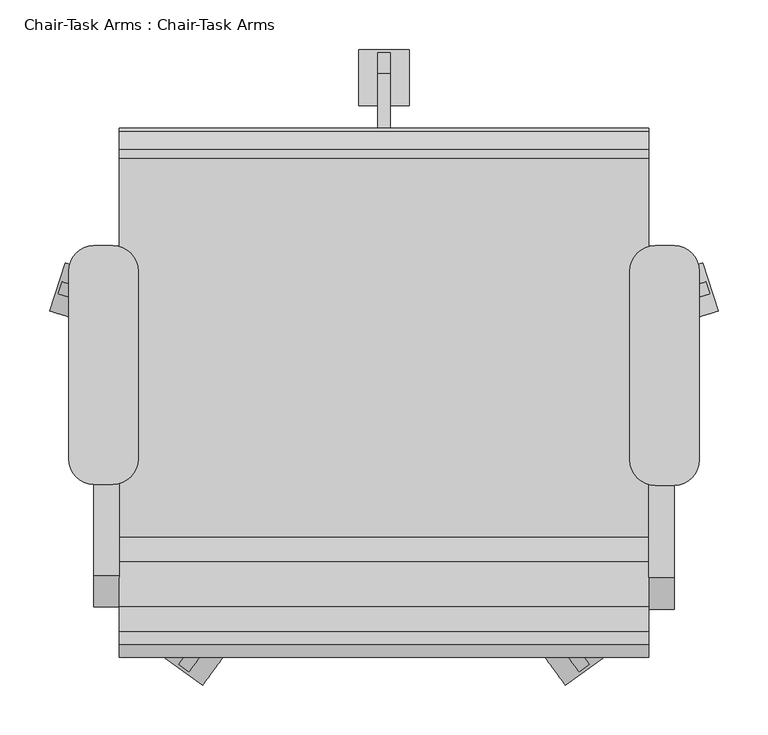
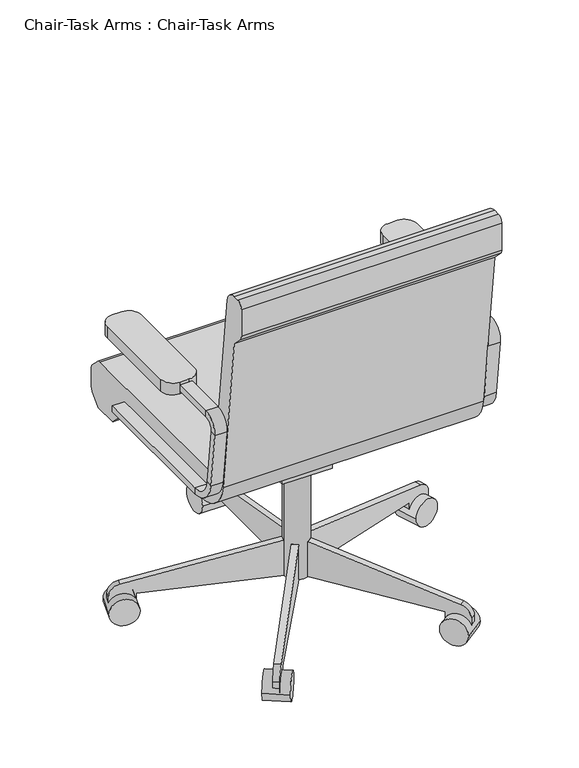
"""IFC4 building model written with IfcOpenShell, lengths in millimetres: furniture geometry, Chair-Task Arms : Chair-Task Arms."""

from ifc_helpers import new_model, si_unit, point, frame, frame_2d, origin, place, context, project, spatial, polyline, circle_curve, trimmed, segment, composite_curve, outline, extrude, source, transform, mapped, element, save
from ifc_brep_helpers import plane_surface, cylinder_surface, revolved_surface, advanced_brep


def chair_task_arms_chair_task_arms_bb362225(model_context):
    return source(origin(), model_context, "Body", "SolidModel", [
        extrude(outline(composite_curve([segment(polyline([(-126.2050455, 457.2), (255.0102301, 457.2)]), True, "CONTINUOUS"), segment(trimmed(circle_curve(frame_2d((255.0102301, 444.5)), 12.7), [point((255.0102301, 457.2))], [point((263.9604301, 453.510212))], False, "CARTESIAN"), True, "CONTINUOUS"), segment(polyline([(263.9604301, 453.510212), (281.8961016, 435.6939999)]), True, "CONTINUOUS"), segment(trimmed(circle_curve(frame_2d((272.9459016, 426.6837879)), 12.7), [point((281.8961016, 435.6939999))], [point((285.6459016, 426.6837879))], False, "CARTESIAN"), True, "CONTINUOUS"), segment(polyline([(285.6459016, 426.6837879), (285.6459016, 391.6405184)]), True, "CONTINUOUS"), segment(trimmed(circle_curve(frame_2d((260.2459016, 391.6405184)), 25.4), [point((285.6459016, 391.6405184))], [point((278.2663256, 373.7401184))], False, "CARTESIAN"), True, "CONTINUOUS"), segment(polyline([(278.2663256, 373.7401184), (260.2470284, 355.6), (209.4470284, 355.6), (181.0744602, 383.7835944), (-107.1089978, 383.7835944)]), True, "CONTINUOUS"), segment(trimmed(circle_curve(frame_2d((-107.1089978, 459.9835944)), 76.2), [point((-107.1089978, 383.7835944))], [point((-182.7870738, 451.0802913))], False, "CARTESIAN"), True, "CONTINUOUS"), segment(polyline([(-182.7870738, 451.0802913), (-222.3540984, 787.4), (-244.0343545, 809.0802561)]), True, "CONTINUOUS"), segment(trimmed(circle_curve(frame_2d((-235.0540984, 818.0605122)), 12.7), [point((-244.0343545, 809.0802561))], [point((-247.7540984, 818.0605122))], False, "CARTESIAN"), True, "CONTINUOUS"), segment(polyline([(-247.7540984, 818.0605122), (-247.7540984, 876.3)]), True, "CONTINUOUS"), segment(trimmed(circle_curve(frame_2d((-235.0540984, 876.3)), 12.7), [point((-247.7540984, 876.3))], [point((-235.0540984, 889.0))], False, "CARTESIAN"), True, "CONTINUOUS"), segment(polyline([(-235.0540984, 889.0), (-222.1789239, 889.0)]), True, "CONTINUOUS"), segment(trimmed(circle_curve(frame_2d((-222.1789239, 863.6)), 25.4), [point((-222.1789239, 889.0))], [point((-196.9528985, 866.5677677))], False, "CARTESIAN"), True, "CONTINUOUS"), segment(polyline([(-196.9528985, 866.5677677), (-151.4310708, 479.6322323)]), True, "CONTINUOUS"), segment(trimmed(circle_curve(frame_2d((-126.2050455, 482.6)), 25.4), [point((-151.4310708, 479.6322323))], [point((-126.2050455, 457.2))], True, "CARTESIAN"), True, "CONTINUOUS")], self_intersect=False)), frame((-125.7091803, 0.0, 0.0), z_axis=(1.0, 0.0, 0.0), x_axis=(0.0, 1.0, 0.0)), (0.0, 0.0, 1.0), 533.4),
        extrude(outline(polyline([(69.7459016, 383.7835944), (69.7459016, 371.0835944), (18.9459016, 283.0954134), (-19.1540984, 283.0954134), (-19.1540984, 383.7835944), (69.7459016, 383.7835944)])), frame((90.1908197, 0.0, 0.0), z_axis=(1.0, 0.0, 0.0), x_axis=(0.0, 1.0, 0.0)), (0.0, 0.0, 1.0), 101.6),
        extrude(outline(composite_curve([segment(polyline([(311.0459016, 53.5835944), (18.9459016, 53.5835944), (18.9459016, 129.7835944), (44.3459016, 129.7835944), (340.8565654, 77.5007643)]), True, "CONTINUOUS"), segment(trimmed(circle_curve(frame_2d((336.4459016, 52.4866474)), 25.4), [point((340.8565654, 77.5007643))], [point((361.8459016, 52.4866474))], False, "CARTESIAN"), True, "CONTINUOUS"), segment(polyline([(361.8459016, 52.4866474), (361.8459016, 28.1835944), (311.0459016, 28.1835944), (311.0459016, 53.5835944)]), True, "CONTINUOUS")], self_intersect=False)), frame((134.6408197, 0.0, 0.0), z_axis=(1.0, 0.0, 0.0), x_axis=(0.0, 1.0, 0.0)), (0.0, 0.0, 1.0), 12.7),
        extrude(outline(composite_curve([segment(trimmed(circle_curve(frame_2d((336.4459016, 28.1835944)), 28.2002727), [point((308.2456289, 28.1835944))], [point((364.6461744, 28.1835944))], False, "CARTESIAN"), True, "CONTINUOUS"), segment(trimmed(circle_curve(frame_2d((336.4459016, 28.1835944)), 28.2002727), [point((364.6461744, 28.1835944))], [point((308.2456289, 28.1835944))], False, "CARTESIAN"), True, "CONTINUOUS")], self_intersect=False)), frame((115.5908197, 0.0, 0.0), z_axis=(1.0, 0.0, 0.0), x_axis=(0.0, 1.0, 0.0)), (0.0, 0.0, 1.0), 50.8),
        extrude(outline(composite_curve([segment(polyline([(25.4, 0.0), (25.4, 292.1000001), (101.6, 292.1000001), (101.6, 266.7), (49.3171699, -29.8106636)]), True, "CONTINUOUS"), segment(trimmed(circle_curve(frame_2d((24.303053, -25.4)), 25.4), [point((49.3171699, -29.8106636))], [point((24.303053, -50.8))], False, "CARTESIAN"), True, "CONTINUOUS"), segment(polyline([(24.303053, -50.8), (0.0, -50.8), (0.0, 0.0), (25.4, 0.0)]), True, "CONTINUOUS")], self_intersect=False)), frame((-138.7750467, 103.1705568, 28.1835944), z_axis=(0.3090169943749487, 0.9510565162951532, 0.0), x_axis=(0.0, 0.0, 1.0)), (0.0, 0.0, 1.0), 12.7),
        extrude(outline(composite_curve([segment(trimmed(circle_curve(frame_2d((0.0, -28.2002727)), 28.2002727), [point((0.0, -56.4005454))], [point((0.0, 0.0))], False, "CARTESIAN"), True, "CONTINUOUS"), segment(trimmed(circle_curve(frame_2d((0.0, -28.2002727)), 28.2002727), [point((0.0, 0.0))], [point((0.0, -56.4005454))], False, "CARTESIAN"), True, "CONTINUOUS")], self_intersect=False)), frame((-195.638709, 101.6163254, 28.1835944), z_axis=(0.3090169943749487, 0.9510565162951532, 0.0), x_axis=(0.0, 0.0, -1.0)), (0.0, 0.0, 1.0), 50.8),
        extrude(outline(composite_curve([segment(polyline([(25.4, 0.0), (25.4, 292.1), (101.6, 292.1), (101.6, 266.7), (49.3171699, -29.8106637)]), True, "CONTINUOUS"), segment(trimmed(circle_curve(frame_2d((24.303053, -25.3999999)), 25.4), [point((49.3171699, -29.8106637))], [point((24.303053, -50.8))], False, "CARTESIAN"), True, "CONTINUOUS"), segment(polyline([(24.303053, -50.8), (0.0, -50.8), (0.0, 0.0), (25.4, 0.0)]), True, "CONTINUOUS")], self_intersect=False)), frame((-25.5639946, -221.1003988, 28.1835944), z_axis=(-0.8090169943749459, 0.5877852522924754, 0.0), x_axis=(0.0, 0.0, 1.0)), (0.0, 0.0, 1.0), 12.7),
        extrude(outline(composite_curve([segment(trimmed(circle_curve(frame_2d((0.0, -28.2002727)), 28.2002727), [point((0.0, -56.4005455))], [point((0.0, 0.0))], False, "CARTESIAN"), True, "CONTINUOUS"), segment(trimmed(circle_curve(frame_2d((0.0, -28.2002727)), 28.2002727), [point((0.0, 0.0))], [point((0.0, -56.4005455))], False, "CARTESIAN"), True, "CONTINUOUS")], self_intersect=False)), frame((-41.6576707, -275.6612394, 28.1835944), z_axis=(-0.8090169943749458, 0.5877852522924754, 0.0), x_axis=(0.0, 0.0, -1.0)), (0.0, 0.0, 1.0), 50.8),
        extrude(outline(composite_curve([segment(polyline([(-25.4, 0.0), (0.0, 0.0), (0.0, -50.8), (-24.303053, -50.8)]), True, "CONTINUOUS"), segment(trimmed(circle_curve(frame_2d((-24.303053, -25.3999999)), 25.4), [point((-24.303053, -50.8))], [point((-49.3171699, -29.8106636))], False, "CARTESIAN"), True, "CONTINUOUS"), segment(polyline([(-49.3171699, -29.8106636), (-101.6, 266.7), (-101.6, 292.1), (-25.4, 292.1), (-25.4, 0.0)]), True, "CONTINUOUS")], self_intersect=False)), frame((307.545634, -221.1003988, 28.1835944), z_axis=(0.8090169943749499, 0.5877852522924699, 0.0), x_axis=(0.0, 0.0, -1.0)), (0.0, 0.0, 1.0), 12.7),
        extrude(outline(composite_curve([segment(trimmed(circle_curve(frame_2d((0.0, -28.2002727)), 28.2002727), [point((0.0, -56.4005455))], [point((0.0, 0.0))], False, "CARTESIAN"), True, "CONTINUOUS"), segment(trimmed(circle_curve(frame_2d((0.0, -28.2002727)), 28.2002727), [point((0.0, 0.0))], [point((0.0, -56.4005455))], False, "CARTESIAN"), True, "CONTINUOUS")], self_intersect=False)), frame((323.63931, -275.6612394, 28.1835944), z_axis=(0.8090169943749499, 0.5877852522924699, 0.0), x_axis=(0.0, 0.0, 1.0)), (0.0, 0.0, 1.0), 50.8),
        extrude(outline(composite_curve([segment(polyline([(-25.4, 0.0), (0.0, 0.0), (0.0, -50.8), (-24.303053, -50.8)]), True, "CONTINUOUS"), segment(trimmed(circle_curve(frame_2d((-24.303053, -25.4)), 25.4), [point((-24.303053, -50.8))], [point((-49.3171699, -29.8106637))], False, "CARTESIAN"), True, "CONTINUOUS"), segment(polyline([(-49.3171699, -29.8106637), (-101.6, 266.7), (-101.6, 292.1), (-25.4, 292.1), (-25.4, 0.0)]), True, "CONTINUOUS")], self_intersect=False)), frame((420.756686, 103.1705568, 28.1835944), z_axis=(-0.3090169943749423, 0.9510565162951553, 0.0), x_axis=(0.0, 0.0, -1.0)), (0.0, 0.0, 1.0), 12.7),
        extrude(outline(composite_curve([segment(trimmed(circle_curve(frame_2d((0.0, -28.2002727)), 28.2002727), [point((0.0, -56.4005455))], [point((0.0, 0.0))], False, "CARTESIAN"), True, "CONTINUOUS"), segment(trimmed(circle_curve(frame_2d((0.0, -28.2002727)), 28.2002727), [point((0.0, 0.0))], [point((0.0, -56.4005455))], False, "CARTESIAN"), True, "CONTINUOUS")], self_intersect=False)), frame((477.6203484, 101.6163254, 28.1835944), z_axis=(-0.3090169943749423, 0.9510565162951553, 0.0), x_axis=(0.0, 0.0, 1.0)), (0.0, 0.0, 1.0), 50.8),
        extrude(outline(composite_curve([segment(trimmed(circle_curve(frame_2d((140.9908197, 18.9459016)), 25.4), [point((115.5908197, 18.9459016))], [point((166.3908197, 18.9459016))], False, "CARTESIAN"), True, "CONTINUOUS"), segment(trimmed(circle_curve(frame_2d((140.9908197, 18.9459016)), 25.4), [point((166.3908197, 18.9459016))], [point((115.5908197, 18.9459016))], False, "CARTESIAN"), True, "CONTINUOUS")], self_intersect=False)), frame((0.0, 0.0, 53.5835944), z_axis=(0.0, 0.0, 1.0), x_axis=(1.0, 0.0, 0.0)), (0.0, 0.0, 1.0), 330.5914056),
        advanced_brep(
        [(433.0908197, 167.0319091, 425.45), (433.0908197, 167.0319091, 412.75), (407.6908197, 167.0319091, 412.75), (407.6908197, 167.0319091, 425.45), (433.0908197, -128.329278, 425.45), (433.0908197, -128.329278, 412.75), (407.6908197, -128.329278, 412.75), (407.6908197, -128.329278, 425.45), (433.0908197, -185.0878351, 463.2225227), (433.0908197, -172.4748224, 464.7064065), (407.6908197, -185.0878351, 463.2225227), (407.6908197, -172.4748224, 464.7064065), (433.0908197, -186.2710303, 581.9741742), (433.0908197, -198.884043, 580.4902904), (407.6908197, -198.884043, 580.4902904), (407.6908197, -186.2710303, 581.9741742), (433.0908197, -167.3515113, 615.95), (433.0908197, -167.3515113, 603.25), (407.6908197, -167.3515113, 615.95), (407.6908197, -167.3515113, 603.25), (433.0908197, 18.9459016, 603.25), (407.6908197, 18.9459016, 603.25), (407.6908197, 18.9459016, 615.95), (433.0908197, 18.9459016, 615.95)],
        [
            (0, 1),
            (1, 2),
            (2, 3),
            (3, 0),
            (0, 4),
            (4, 5),
            (5, 1),
            (5, 6),
            (6, 2),
            (6, 7),
            (7, 3),
            (7, 4),
            (8, 5, circle_curve(frame((433.0908197, -128.329278, 469.9), z_axis=(1.0, 0.0, 0.0), x_axis=(0.0, 0.0, -1.0)), 57.15)),
            (4, 9, circle_curve(frame((433.0908197, -128.329278, 469.9), z_axis=(-1.0, 0.0, 0.0), x_axis=(0.0, 0.0, -1.0)), 44.45)),
            (9, 8),
            (10, 6, circle_curve(frame((407.6908197, -128.329278, 469.9), z_axis=(1.0, 0.0, 0.0), x_axis=(0.0, 0.0, -1.0)), 57.15)),
            (8, 10),
            (11, 7, circle_curve(frame((407.6908197, -128.329278, 469.9), z_axis=(1.0, 0.0, 0.0), x_axis=(0.0, 0.0, -1.0)), 44.45)),
            (10, 11),
            (11, 9),
            (9, 12),
            (12, 13),
            (13, 8),
            (13, 14),
            (14, 10),
            (14, 15),
            (15, 11),
            (15, 12),
            (16, 13, circle_curve(frame((433.0908197, -167.3515113, 584.2), z_axis=(1.0, 0.0, 0.0), x_axis=(0.0, -0.9931506043228767, -0.1168412475673929)), 31.75)),
            (12, 17, circle_curve(frame((433.0908197, -167.3515113, 584.2), z_axis=(-1.0, 0.0, 0.0), x_axis=(0.0, -0.9931506043228767, -0.1168412475673929)), 19.05)),
            (17, 16),
            (18, 14, circle_curve(frame((407.6908197, -167.3515113, 584.2), z_axis=(1.0, 0.0, 0.0), x_axis=(0.0, -0.9931506043228767, -0.1168412475673929)), 31.75)),
            (16, 18),
            (19, 15, circle_curve(frame((407.6908197, -167.3515113, 584.2), z_axis=(1.0, 0.0, 0.0), x_axis=(0.0, -0.9931506043228767, -0.1168412475673929)), 19.05)),
            (18, 19),
            (19, 17),
            (20, 21),
            (21, 22),
            (22, 23),
            (23, 20),
            (17, 20),
            (23, 16),
            (22, 18),
            (21, 19),
        ],
        [
            plane_surface(frame((406.191788, 167.0319091, 419.1), z_axis=(0.0, 1.0, 0.0), x_axis=(0.0, 0.0, -1.0))),
            plane_surface(frame((433.0908197, 167.0319091, 425.45), z_axis=(1.0, 0.0, 0.0), x_axis=(0.0, -1.0, 0.0))),
            plane_surface(frame((433.0908197, 167.0319091, 412.75), z_axis=(0.0, 0.0, -1.0), x_axis=(0.0, -1.0, 0.0))),
            plane_surface(frame((407.6908197, 167.0319091, 412.75), z_axis=(-1.0, 0.0, 0.0), x_axis=(0.0, -1.0, 0.0))),
            plane_surface(frame((407.6908197, 167.0319091, 425.45), z_axis=(0.0, 0.0, 1.0), x_axis=(0.0, -1.0, 0.0))),
            plane_surface(frame((433.0908197, -128.329278, 469.9), z_axis=(1.0, 0.0, 0.0), x_axis=(0.0, 0.0, -1.0))),
            cylinder_surface(frame((420.3908197, -128.329278, 469.9), z_axis=(-1.0, 0.0, 0.0), x_axis=(0.0, 0.0, -1.0)), 57.15),
            plane_surface(frame((407.6908197, -128.329278, 469.9), z_axis=(-1.0, 0.0, 0.0), x_axis=(0.0, 0.0, -1.0))),
            revolved_surface(polyline([(407.6908197, -128.329278, 425.45), (433.0908197, -128.329278, 425.45)]), (420.3908197, -128.329278, 469.9), (-1.0, 0.0, 0.0)),
            plane_surface(frame((433.0908197, -172.4748224, 464.7064065), z_axis=(1.0, 0.0, 0.0), x_axis=(0.0, -0.11684124756738626, 0.9931506043228775))),
            plane_surface(frame((433.0908197, -185.0878351, 463.2225227), z_axis=(0.0, -0.9931506043228775, -0.11684124756738655), x_axis=(0.0, -0.11684124756738655, 0.9931506043228775))),
            plane_surface(frame((407.6908197, -185.0878351, 463.2225227), z_axis=(-1.0, 0.0, 0.0), x_axis=(0.0, -0.11684124756738626, 0.9931506043228775))),
            plane_surface(frame((407.6908197, -172.4748224, 464.7064065), z_axis=(0.0, 0.9931506043228775, 0.11684124756738626), x_axis=(0.0, -0.11684124756738626, 0.9931506043228775))),
            plane_surface(frame((433.0908197, -167.3515113, 584.2), z_axis=(1.0, 0.0, 0.0), x_axis=(0.0, -0.9931506043228767, -0.1168412475673929))),
            cylinder_surface(frame((420.3908197, -167.3515113, 584.2), z_axis=(-1.0, 0.0, 0.0), x_axis=(0.0, -0.9931506043228767, -0.1168412475673929)), 31.75),
            plane_surface(frame((407.6908197, -167.3515113, 584.2), z_axis=(-1.0, 0.0, 0.0), x_axis=(0.0, -0.9931506043228767, -0.1168412475673929))),
            revolved_surface(polyline([(407.6908197, -186.2710303123508, 581.9741742338412), (433.0908197, -186.2710303123508, 581.9741742338412)]), (420.3908197, -167.3515113, 584.2), (-1.0, 0.0, 0.0)),
            plane_surface(frame((406.191788, 18.9459016, 609.6), z_axis=(0.0, 1.0, 0.0), x_axis=(0.0, 0.0, 1.0))),
            plane_surface(frame((433.0908197, -167.3515113, 603.25), z_axis=(1.0, 0.0, 0.0), x_axis=(0.0, 1.0, 0.0))),
            plane_surface(frame((433.0908197, -167.3515113, 615.95), z_axis=(0.0, 0.0, 1.0), x_axis=(0.0, 1.0, 0.0))),
            plane_surface(frame((407.6908197, -167.3515113, 615.95), z_axis=(-1.0, 0.0, 0.0), x_axis=(0.0, 1.0, 0.0))),
            plane_surface(frame((407.6908197, -167.3515113, 603.25), z_axis=(0.0, 0.0, -1.0), x_axis=(0.0, 1.0, 0.0))),
        ],
        [
            (0, [[1, 2, 3, 4]]),
            (1, [[-1, 5, 6, 7]]),
            (2, [[-2, -7, 8, 9]]),
            (3, [[-3, -9, 10, 11]]),
            (4, [[-4, -11, 12, -5]]),
            (5, [[13, -6, 14, 15]]),
            (6, [[16, -8, -13, 17]]),
            (7, [[18, -10, -16, 19]]),
            (8, [[-14, -12, -18, 20]]),
            (9, [[-15, 21, 22, 23]]),
            (10, [[-17, -23, 24, 25]]),
            (11, [[-19, -25, 26, 27]]),
            (12, [[-20, -27, 28, -21]]),
            (13, [[29, -22, 30, 31]]),
            (14, [[32, -24, -29, 33]]),
            (15, [[34, -26, -32, 35]]),
            (16, [[-30, -28, -34, 36]]),
            (17, [[37, 38, 39, 40]]),
            (18, [[-31, 41, -40, 42]]),
            (19, [[-33, -42, -39, 43]]),
            (20, [[-35, -43, -38, 44]]),
            (21, [[-36, -44, -37, -41]]),
        ],
    ),
        advanced_brep(
        [(-151.1091803, 167.0319091, 412.75), (-151.1091803, 167.0319091, 425.45), (-125.7091803, 167.0319091, 425.45), (-125.7091803, 167.0319091, 412.75), (-151.1091803, -126.2388651, 412.75), (-151.1091803, -126.2388651, 425.45), (-125.7091803, -126.2388651, 425.45), (-125.7091803, -126.2388651, 412.75), (-151.1091803, -170.3844094, 464.7064065), (-151.1091803, -182.9974221, 463.2225227), (-125.7091803, -170.3844094, 464.7064065), (-125.7091803, -182.9974221, 463.2225227), (-151.1091803, -196.7936301, 580.4902904), (-151.1091803, -184.1806174, 581.9741742), (-125.7091803, -184.1806174, 581.9741742), (-125.7091803, -196.7936301, 580.4902904), (-151.1091803, -165.2610984, 603.25), (-151.1091803, -165.2610984, 615.95), (-125.7091803, -165.2610984, 603.25), (-125.7091803, -165.2610984, 615.95), (-151.1091803, 18.9459016, 615.95), (-125.7091803, 18.9459016, 615.95), (-125.7091803, 18.9459016, 603.25), (-151.1091803, 18.9459016, 603.25)],
        [
            (0, 1),
            (1, 2),
            (2, 3),
            (3, 0),
            (0, 4),
            (4, 5),
            (5, 1),
            (5, 6),
            (6, 2),
            (6, 7),
            (7, 3),
            (7, 4),
            (8, 5, circle_curve(frame((-151.1091803, -126.2388651, 469.9), z_axis=(1.0, 0.0, 0.0), x_axis=(0.0, 0.0, -1.0)), 44.45)),
            (4, 9, circle_curve(frame((-151.1091803, -126.2388651, 469.9), z_axis=(-1.0, 0.0, 0.0), x_axis=(0.0, 0.0, -1.0)), 57.15)),
            (9, 8),
            (10, 6, circle_curve(frame((-125.7091803, -126.2388651, 469.9), z_axis=(1.0, 0.0, 0.0), x_axis=(0.0, 0.0, -1.0)), 44.45)),
            (8, 10),
            (11, 7, circle_curve(frame((-125.7091803, -126.2388651, 469.9), z_axis=(1.0, 0.0, 0.0), x_axis=(0.0, 0.0, -1.0)), 57.15)),
            (10, 11),
            (11, 9),
            (9, 12),
            (12, 13),
            (13, 8),
            (13, 14),
            (14, 10),
            (14, 15),
            (15, 11),
            (15, 12),
            (16, 13, circle_curve(frame((-151.1091803, -165.2610984, 584.2), z_axis=(1.0, 0.0, 0.0), x_axis=(0.0, -0.9931506043228768, -0.11684124756739202)), 19.05)),
            (12, 17, circle_curve(frame((-151.1091803, -165.2610984, 584.2), z_axis=(-1.0, 0.0, 0.0), x_axis=(0.0, -0.9931506043228768, -0.11684124756739202)), 31.75)),
            (17, 16),
            (18, 14, circle_curve(frame((-125.7091803, -165.2610984, 584.2), z_axis=(1.0, 0.0, 0.0), x_axis=(0.0, -0.9931506043228768, -0.11684124756739202)), 19.05)),
            (16, 18),
            (19, 15, circle_curve(frame((-125.7091803, -165.2610984, 584.2), z_axis=(1.0, 0.0, 0.0), x_axis=(0.0, -0.9931506043228768, -0.11684124756739202)), 31.75)),
            (18, 19),
            (19, 17),
            (20, 21),
            (21, 22),
            (22, 23),
            (23, 20),
            (17, 20),
            (23, 16),
            (22, 18),
            (21, 19),
        ],
        [
            plane_surface(frame((-152.608212, 167.0319091, 419.1), z_axis=(0.0, 1.0, 0.0), x_axis=(0.0, 0.0, -1.0))),
            plane_surface(frame((-151.1091803, 167.0319091, 412.75), z_axis=(-1.0, 0.0, 0.0), x_axis=(0.0, -1.0, 0.0))),
            plane_surface(frame((-151.1091803, 167.0319091, 425.45), z_axis=(0.0, 0.0, 1.0), x_axis=(0.0, -1.0, 0.0))),
            plane_surface(frame((-125.7091803, 167.0319091, 425.45), z_axis=(1.0, 0.0, 0.0), x_axis=(0.0, -1.0, 0.0))),
            plane_surface(frame((-125.7091803, 167.0319091, 412.75), z_axis=(0.0, 0.0, -1.0), x_axis=(0.0, -1.0, 0.0))),
            plane_surface(frame((-151.1091803, -126.2388651, 469.9), z_axis=(-1.0, 0.0, 0.0), x_axis=(0.0, 0.0, -1.0))),
            revolved_surface(polyline([(-151.1091803, -126.2388651, 425.45), (-125.7091803, -126.2388651, 425.45)]), (-138.4091803, -126.2388651, 469.9), (-1.0, 0.0, 0.0)),
            plane_surface(frame((-125.7091803, -126.2388651, 469.9), z_axis=(1.0, 0.0, 0.0), x_axis=(0.0, 0.0, -1.0))),
            cylinder_surface(frame((-138.4091803, -126.2388651, 469.9), z_axis=(-1.0, 0.0, 0.0), x_axis=(0.0, 0.0, -1.0)), 57.15),
            plane_surface(frame((-151.1091803, -182.9974221, 463.2225227), z_axis=(-1.0, 0.0, 0.0), x_axis=(0.0, -0.1168412475673856, 0.9931506043228776))),
            plane_surface(frame((-151.1091803, -170.3844094, 464.7064065), z_axis=(0.0, 0.9931506043228776, 0.1168412475673856), x_axis=(0.0, -0.1168412475673856, 0.9931506043228776))),
            plane_surface(frame((-125.7091803, -170.3844094, 464.7064065), z_axis=(1.0, 0.0, 0.0), x_axis=(0.0, -0.1168412475673856, 0.9931506043228776))),
            plane_surface(frame((-125.7091803, -182.9974221, 463.2225227), z_axis=(0.0, -0.9931506043228776, -0.1168412475673856), x_axis=(0.0, -0.1168412475673856, 0.9931506043228776))),
            plane_surface(frame((-151.1091803, -165.2610984, 584.2), z_axis=(-1.0, 0.0, 0.0), x_axis=(0.0, -0.9931506043228768, -0.11684124756739202))),
            revolved_surface(polyline([(-151.1091803, -184.1806174123508, 581.9741742338413), (-125.7091803, -184.1806174123508, 581.9741742338413)]), (-138.4091803, -165.2610984, 584.2), (-1.0, 0.0, 0.0)),
            plane_surface(frame((-125.7091803, -165.2610984, 584.2), z_axis=(1.0, 0.0, 0.0), x_axis=(0.0, -0.9931506043228768, -0.11684124756739202))),
            cylinder_surface(frame((-138.4091803, -165.2610984, 584.2), z_axis=(-1.0, 0.0, 0.0), x_axis=(0.0, -0.9931506043228768, -0.11684124756739202)), 31.75),
            plane_surface(frame((-152.608212, 18.9459016, 609.6), z_axis=(0.0, 1.0, 0.0), x_axis=(0.0, 0.0, 1.0))),
            plane_surface(frame((-151.1091803, -165.2610984, 615.95), z_axis=(-1.0, 0.0, 0.0), x_axis=(0.0, 1.0, 0.0))),
            plane_surface(frame((-151.1091803, -165.2610984, 603.25), z_axis=(0.0, 0.0, -1.0), x_axis=(0.0, 1.0, 0.0))),
            plane_surface(frame((-125.7091803, -165.2610984, 603.25), z_axis=(1.0, 0.0, 0.0), x_axis=(0.0, 1.0, 0.0))),
            plane_surface(frame((-125.7091803, -165.2610984, 615.95), z_axis=(0.0, 0.0, 1.0), x_axis=(0.0, 1.0, 0.0))),
        ],
        [
            (0, [[1, 2, 3, 4]]),
            (1, [[-1, 5, 6, 7]]),
            (2, [[-2, -7, 8, 9]]),
            (3, [[-3, -9, 10, 11]]),
            (4, [[-4, -11, 12, -5]]),
            (5, [[13, -6, 14, 15]]),
            (6, [[16, -8, -13, 17]]),
            (7, [[18, -10, -16, 19]]),
            (8, [[-14, -12, -18, 20]]),
            (9, [[-15, 21, 22, 23]]),
            (10, [[-17, -23, 24, 25]]),
            (11, [[-19, -25, 26, 27]]),
            (12, [[-20, -27, 28, -21]]),
            (13, [[29, -22, 30, 31]]),
            (14, [[32, -24, -29, 33]]),
            (15, [[34, -26, -32, 35]]),
            (16, [[-30, -28, -34, 36]]),
            (17, [[37, 38, 39, 40]]),
            (18, [[-31, 41, -40, 42]]),
            (19, [[-33, -42, -39, 43]]),
            (20, [[-35, -43, -38, 44]]),
            (21, [[-36, -44, -37, -41]]),
        ],
    ),
        extrude(outline(composite_curve([segment(polyline([(433.0908197, -74.2028048), (414.0408197, -74.2028048)]), True, "CONTINUOUS"), segment(trimmed(circle_curve(frame_2d((414.0408197, -48.8028048)), 25.4), [point((414.0408197, -74.2028048))], [point((388.6408197, -48.8028048))], False, "CARTESIAN"), True, "CONTINUOUS"), segment(polyline([(388.6408197, -48.8028048), (388.6408197, 141.6319091)]), True, "CONTINUOUS"), segment(trimmed(circle_curve(frame_2d((414.0408197, 141.6319091)), 25.4), [point((388.6408197, 141.6319091))], [point((414.0408197, 167.0319091))], False, "CARTESIAN"), True, "CONTINUOUS"), segment(polyline([(414.0408197, 167.0319091), (433.0908197, 167.0319091)]), True, "CONTINUOUS"), segment(trimmed(circle_curve(frame_2d((433.0908197, 141.6319091)), 25.4), [point((433.0908197, 167.0319091))], [point((458.4908197, 141.6319091))], False, "CARTESIAN"), True, "CONTINUOUS"), segment(polyline([(458.4908197, 141.6319091), (458.4908197, -48.8028048)]), True, "CONTINUOUS"), segment(trimmed(circle_curve(frame_2d((433.0908197, -48.8028048)), 25.4), [point((458.4908197, -48.8028048))], [point((433.0908197, -74.2028048))], False, "CARTESIAN"), True, "CONTINUOUS")], self_intersect=False)), frame((0.0, 0.0, 596.9), z_axis=(0.0, 0.0, 1.0), x_axis=(1.0, 0.0, 0.0)), (0.0, 0.0, 1.0), 25.4),
        extrude(outline(composite_curve([segment(polyline([(-132.0591803, -73.1575984), (-151.1091803, -73.1575984)]), True, "CONTINUOUS"), segment(trimmed(circle_curve(frame_2d((-151.1091803, -47.7575984)), 25.4), [point((-151.1091803, -73.1575984))], [point((-176.5091803, -47.7575984))], False, "CARTESIAN"), True, "CONTINUOUS"), segment(polyline([(-176.5091803, -47.7575984), (-176.5091803, 141.6319091)]), True, "CONTINUOUS"), segment(trimmed(circle_curve(frame_2d((-151.1091803, 141.6319091)), 25.4), [point((-176.5091803, 141.6319091))], [point((-151.1091803, 167.0319091))], False, "CARTESIAN"), True, "CONTINUOUS"), segment(polyline([(-151.1091803, 167.0319091), (-132.0591803, 167.0319091)]), True, "CONTINUOUS"), segment(trimmed(circle_curve(frame_2d((-132.0591803, 141.6319091)), 25.4), [point((-132.0591803, 167.0319091))], [point((-106.6591803, 141.6319091))], False, "CARTESIAN"), True, "CONTINUOUS"), segment(polyline([(-106.6591803, 141.6319091), (-106.6591803, -47.7575984)]), True, "CONTINUOUS"), segment(trimmed(circle_curve(frame_2d((-132.0591803, -47.7575984)), 25.4), [point((-106.6591803, -47.7575984))], [point((-132.0591803, -73.1575984))], False, "CARTESIAN"), True, "CONTINUOUS")], self_intersect=False)), frame((0.0, 0.0, 596.9), z_axis=(0.0, 0.0, 1.0), x_axis=(1.0, 0.0, 0.0)), (0.0, 0.0, 1.0), 25.4),
    ])


if __name__ == "__main__":
    model = new_model("IFC4")
    model_context = context("Model", 3, world=origin())
    ifc_project = project(units=[si_unit("LENGTHUNIT", "METRE", prefix="MILLI")], contexts=[model_context])
    site = spatial("IfcSite", under=ifc_project)
    building = spatial("IfcBuilding", under=site)
    placement = place(None, origin())
    chair_task_arms_chair_task_arms_shape = chair_task_arms_chair_task_arms_bb362225(model_context)
    element("IfcFurniture", 1, ObjectType="Chair-Task Arms : Chair-Task Arms", at=placement, inside=building, context=model_context, shape_type="MappedRepresentation", body=[
        mapped(chair_task_arms_chair_task_arms_shape, transform((0.0, 0.0, 0.0), x_axis=(1.0, 0.0, 0.0), y_axis=(0.0, 1.0, 0.0), z_axis=(0.0, 0.0, 1.0))),
    ])
    save(model, "model.ifc")

# Revit data of these elements
# Type "Chair-Task Arms : Chair-Task Arms"
#   Assembly Code = "E2020200"
#   Base Material = Plastic, Opaque Black
#   Caster Material = Plastic, Opaque Black
#   Seat/Back Material = Textile - Slate Blue
#   Default Elevation = 0
# Element 1 (IfcFurniture, "Chair-Task Arms : Chair-Task Arms")
#   Materials on its faces: "Plastic, Opaque Black", "Textile - Slate Blue"
# Materials
#   "Plastic, Opaque Black": class "Plastic", colour RGB 0 0 0, transparency 0.7, Description = "Plastic, generic, opaque black", Cost = 0
#   "Textile - Slate Blue": class "Fabric", colour RGB 98 102 118, transparency 0
